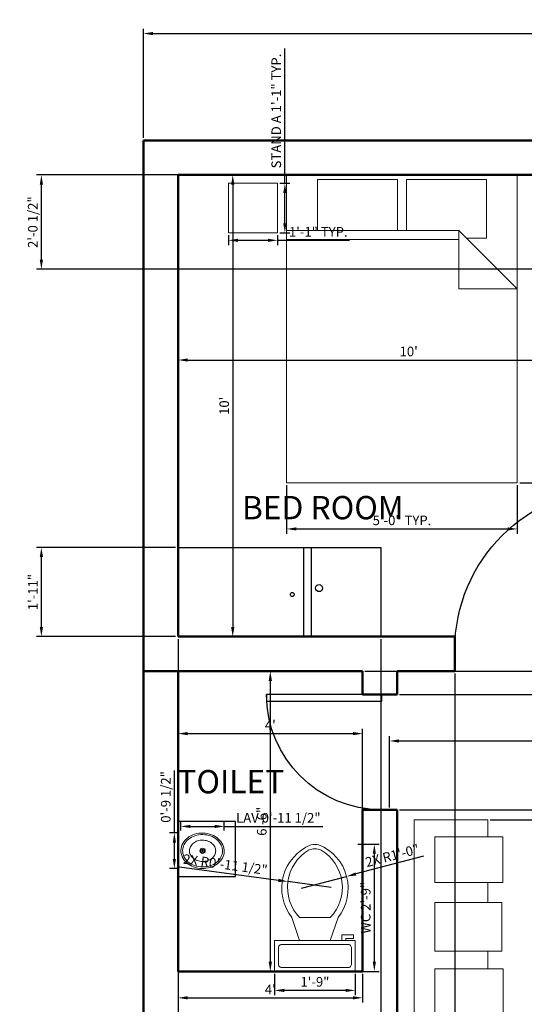
# Model space of a CAD drawing. Units: inches. Extents: x 1071 to 1348, y 2363 to 2916.
# Tile 2 of 4: x 1071 to 1202, y 2660 to 2916. Entities that reach past the tile are written whole.
import ezdxf

# ---------------------------------------------------------------- set-up
doc = ezdxf.new("R2010")
doc.units = ezdxf.units.IN
for name, color, linetype, lineweight in [('A-ANNO-DIMS', 2, 'Continuous', 18), ('A-AREA-IDEN', 7, 'Continuous', 25), ('A-DOOR', 4, 'Continuous', 25), ('A-FLOR-CASE', 9, 'Continuous', 25), ('A-FLOR-FIXT', 9, 'Continuous', 20), ('A-FURN', 8, 'Continuous', 18), ('A-WALL', 7, 'Continuous', 50)]:
    doc.layers.add(name, color=color, linetype=linetype, lineweight=lineweight)
doc.styles.get("Standard").update_dxf_attribs({"font": 'arial.ttf'})
doc.dimstyles.new('ISO-25', dxfattribs={"dimtxt": 2.5, "dimasz": 2.5, "dimexe": 1.25, "dimexo": 0.625, "dimtad": 1, "dimdec": 0, "dimlunit": 3, "dimtxsty": 'Standard', "dimcen": 2.5, "dimadec": 0, "dimazin": 0, "dimtfac": 1, "dimtdec": 0, "dimtmove": 0, "dimatfit": 3, "dimfxl": 1, "dimarcsym": 0})

# ---------------------------------------------------------------- blocks, each defined once
blk = doc.blocks.new('*U2')
for p, q in [((0, 0), (0, -100)), ((750, 0), (750, -100))]:
    blk.add_line(p, q)
blk.add_lwpolyline([(0, 0), (0, 750), (43.75, 750), (43.75, 0)], close=True)
blk.add_arc((0, 0), 750, 0, 90)
blk = doc.blocks.new('Toilet - top')
for p, q in [((9.5, -6), (9.5, -2)), ((-10, -8.5), (-8, -8.5)), ((-10, -9.5), (-10, -8.5)), ((-7, -9.5), (-10, -9.5)), ((-8, -8.5), (-8, -8)), ((-7, -8), (-7, -9.5)), ((-4, -8), (-6, -14)), ((4, -8), (6, -14)), ((4, -14), (-4, -14))]:
    blk.add_line(p, q)
blk.add_lwpolyline([(10.5, -8), (10.5, 0), (-10.5, 0), (-10.5, -8)], close=True)
for points in [[(-9.5, -2), (-9.5, -6)], [(8.5, -1), (-8.5, -1)], [(-8.5, -7), (8.5, -7)]]:
    blk.add_lwpolyline(points)
for centre, radius, start, end in [((-8.62, -1.88), 0.884, 81.8699, 188.1301), ((8.62, -1.88), 0.884, 351.8699, 98.1301), ((-8.62, -6.12), 0.884, 171.8699, 278.1301), ((8.62, -6.12), 0.884, 261.8699, 8.1301), ((3.52, -21.58), 12.17, 141.4691, 247.9714), ((4.2, -21.82), 11.33, 136.3677, 238.9468), ((-3.52, -21.58), 12.17, 292.0284, 38.5307), ((-4.2, -21.82), 11.33, 301.053, 43.6321), ((0, -27.88), 4, 245.7318, 294.2682), ((0, -29), 4, 254.8605, 285.1395)]:
    blk.add_arc(centre, radius, start, end)
blk = doc.blocks.new('Sink - Oval top')
for p, q in [((-1, 0), (1, 0)), ((0, 1), (0, -1))]:
    blk.add_line(p, q)
for points in [[(-12.23, 0.39, 0.117634), (-11.46, -3.36, 0.104469), (-8.88, -6.8, 0.090016), (-5.08, -9.07, 0.08192), (-0.32, -10.02, 0.08192), (4.49, -9.38, 0.090016), (8.42, -7.36, 0.104469), (11.22, -4.09, 0.117634), (12.23, -0.39, 0.117634), (11.46, 3.36, 0.104469), (8.88, 6.8, 0.090016), (5.08, 9.07, 0.08192), (0.32, 10.02, 0.08192), (-4.49, 9.38, 0.090016), (-8.42, 7.36, 0.104469), (-11.22, 4.09, 0.117634)], [(-11.29, 0.16, 0.118622), (-10.52, -3.25, 0.104678), (-8.07, -6.36, 0.089562), (-4.54, -8.37, 0.081185), (-0.13, -9.15, 0.081185), (4.3, -8.49, 0.089562), (7.89, -6.58, 0.104678), (10.42, -3.55, 0.118622), (11.29, -0.16, 0.118622), (10.52, 3.25, 0.104678), (8.07, 6.36, 0.089562), (4.54, 8.37, 0.081185), (0.13, 9.15, 0.081185), (-4.3, 8.49, 0.089562), (-7.89, 6.58, 0.104678), (-10.42, 3.55, 0.118622)], [(-7.42, 0.08, 0.118283), (-6.91, -2.17, 0.104607), (-5.29, -4.21, 0.089718), (-2.97, -5.53, 0.081436), (-0.07, -6.04, 0.081436), (2.84, -5.59, 0.089718), (5.2, -4.33, 0.104607), (6.86, -2.32, 0.118283), (7.42, -0.08, 0.118283), (6.91, 2.17, 0.104607), (5.29, 4.21, 0.089718), (2.97, 5.53, 0.081436), (0.07, 6.04, 0.081436), (-2.84, 5.59, 0.089718), (-5.2, 4.33, 0.104607), (-6.86, 2.32, 0.118283)]]:
    blk.add_lwpolyline(points, format="xyb", close=True)
for radius in [1.5, 1]:
    blk.add_circle((0, 0), radius)
blk = doc.blocks.new('Bed - Queen')
for p, q in [((0, -80.00003), (0, 0)), ((0, 0), (59.99999, 0)), ((59.99999, 0), (59.99999, -80.00003)), ((7.99999, -1.2), (28.79998, -1.2)), ((7.99999, -14.4), (7.99999, -1.2)), ((28.79998, -1.2), (28.79998, -14.4)), ((31.19999, -1.2), (51.99999, -1.2)), ((31.19999, -14.4), (31.19999, -1.2)), ((51.99999, -1.2), (51.99999, -16.4)), ((0, -14.4), (44.8, -14.4)), ((59.99999, -29.6), (44.8, -14.4)), ((44.8, -14.4), (44.8, -29.6)), ((44.8, -16.8), (0, -16.8)), ((51.99999, -16.4), (46.79936, -16.4)), ((44.8, -29.6), (59.99999, -29.6)), ((59.99999, -80.00003), (0, -80.00003))]:
    blk.add_line(p, q)
blk = doc.blocks.new('*D9')
at = {"layer": 'A-ANNO-DIMS', "color": 0, "lineweight": -2, "transparency": 16777216}
for p, q in [((1103.28, 2884.88), (1103.28, 2913.26)), ((1319.28, 2884.88), (1319.28, 2913.26)), ((1105.78, 2912.01), (1316.78, 2912.01))]:
    blk.add_line(p, q, dxfattribs=at)
at = {"layer": 'A-ANNO-DIMS', "color": 0, "transparency": 16777216}
for points in [[(1105.78, 2912.43), (1105.78, 2911.6), (1103.28, 2912.01)], [(1316.78, 2912.43), (1316.78, 2911.6), (1319.28, 2912.01)]]:
    blk.add_solid(points, dxfattribs=at)
at = {"layer": 'Defpoints', "color": 0, "transparency": 16777216}
for p in [(1319.28, 2912.01), (1103.28, 2884.25), (1319.28, 2884.25)]:
    blk.add_point(p, dxfattribs=at)
at = {"layer": 'A-ANNO-DIMS', "color": 0, "transparency": 16777216, "insert": (1211.28, 2913.91), "char_height": 2.5, "attachment_point": 5}
blk.add_mtext("18'", dxfattribs=at)
blk = doc.blocks.new('*D14')
at = {"layer": 'A-ANNO-DIMS', "color": 0, "lineweight": -2, "transparency": 16777216}
for p, q in [((1167.28, 2710.88), (1167.28, 2729.38)), ((1310.28, 2710.88), (1310.28, 2729.38)), ((1169.78, 2728.13), (1307.78, 2728.13))]:
    blk.add_line(p, q, dxfattribs=at)
at = {"layer": 'A-ANNO-DIMS', "color": 0, "transparency": 16777216}
for points in [[(1169.78, 2728.55), (1169.78, 2727.72), (1167.28, 2728.13)], [(1307.78, 2728.55), (1307.78, 2727.72), (1310.28, 2728.13)]]:
    blk.add_solid(points, dxfattribs=at)
at = {"layer": 'Defpoints', "color": 0, "transparency": 16777216}
for p in [(1310.28, 2728.13), (1167.28, 2710.25), (1310.28, 2710.25)]:
    blk.add_point(p, dxfattribs=at)
at = {"layer": 'A-ANNO-DIMS', "color": 0, "transparency": 16777216, "insert": (1238.78, 2730.01), "char_height": 2.5, "attachment_point": 5}
blk.add_mtext('11\'-11"', dxfattribs=at)
blk = doc.blocks.new('*D19')
at = {"layer": 'A-ANNO-DIMS', "color": 0, "lineweight": -2, "transparency": 16777216}
for p, q in [((1112.91, 2746.25), (1137.53, 2746.25)), ((1136.28, 2743.75), (1136.28, 2670.75)), ((1112.91, 2668.25), (1137.53, 2668.25))]:
    blk.add_line(p, q, dxfattribs=at)
at = {"layer": 'A-ANNO-DIMS', "color": 0, "transparency": 16777216}
for points in [[(1135.86, 2743.75), (1136.7, 2743.75), (1136.28, 2746.25)], [(1135.86, 2670.75), (1136.7, 2670.75), (1136.28, 2668.25)]]:
    blk.add_solid(points, dxfattribs=at)
at = {"layer": 'Defpoints', "color": 0, "transparency": 16777216}
for p in [(1112.28, 2746.25), (1112.28, 2668.25), (1136.28, 2668.25)]:
    blk.add_point(p, dxfattribs=at)
at = {"layer": 'A-ANNO-DIMS', "color": 0, "transparency": 16777216, "insert": (1134.38, 2707.25), "char_height": 2.5, "attachment_point": 5, "rotation": 90}
blk.add_mtext('6\'-6"', dxfattribs=at)
blk = doc.blocks.new('*D20')
at = {"layer": 'A-ANNO-DIMS', "color": 0, "lineweight": -2, "transparency": 16777216}
for p, q in [((1112.28, 2668.88), (1112.28, 2731.3)), ((1160.28, 2668.88), (1160.28, 2731.3)), ((1114.78, 2730.05), (1157.78, 2730.05))]:
    blk.add_line(p, q, dxfattribs=at)
at = {"layer": 'A-ANNO-DIMS', "color": 0, "transparency": 16777216}
for points in [[(1114.78, 2730.47), (1114.78, 2729.63), (1112.28, 2730.05)], [(1157.78, 2730.47), (1157.78, 2729.63), (1160.28, 2730.05)]]:
    blk.add_solid(points, dxfattribs=at)
at = {"layer": 'Defpoints', "color": 0, "transparency": 16777216}
for p in [(1160.28, 2730.05), (1112.28, 2668.25), (1160.28, 2668.25)]:
    blk.add_point(p, dxfattribs=at)
at = {"layer": 'A-ANNO-DIMS', "color": 0, "transparency": 16777216, "insert": (1136.28, 2731.93), "char_height": 2.5, "attachment_point": 5}
blk.add_mtext("4'", dxfattribs=at)
blk = doc.blocks.new('*D24')
at = {"layer": 'A-ANNO-DIMS', "color": 0, "lineweight": -2, "transparency": 16777216}
for p, q in [((1112.28, 2874.63), (1112.28, 2825.9)), ((1232.28, 2874.63), (1232.28, 2825.9)), ((1114.78, 2827.15), (1229.78, 2827.15))]:
    blk.add_line(p, q, dxfattribs=at)
at = {"layer": 'A-ANNO-DIMS', "color": 0, "transparency": 16777216}
for points in [[(1114.78, 2827.57), (1114.78, 2826.74), (1112.28, 2827.15)], [(1229.78, 2827.57), (1229.78, 2826.74), (1232.28, 2827.15)]]:
    blk.add_solid(points, dxfattribs=at)
at = {"layer": 'Defpoints', "color": 0, "transparency": 16777216}
for p in [(1112.28, 2875.25), (1232.28, 2875.25), (1232.28, 2827.15)]:
    blk.add_point(p, dxfattribs=at)
at = {"layer": 'A-ANNO-DIMS', "color": 0, "transparency": 16777216, "insert": (1172.28, 2829.06), "char_height": 2.5, "attachment_point": 5}
blk.add_mtext("10'", dxfattribs=at)
blk = doc.blocks.new('*D25')
at = {"layer": 'A-ANNO-DIMS', "color": 0, "lineweight": -2, "transparency": 16777216}
for p, q in [((1112.91, 2875.25), (1127.76, 2875.25)), ((1126.51, 2872.75), (1126.51, 2757.75)), ((1112.91, 2755.25), (1127.76, 2755.25))]:
    blk.add_line(p, q, dxfattribs=at)
at = {"layer": 'A-ANNO-DIMS', "color": 0, "transparency": 16777216}
for points in [[(1126.09, 2872.75), (1126.93, 2872.75), (1126.51, 2875.25)], [(1126.09, 2757.75), (1126.93, 2757.75), (1126.51, 2755.25)]]:
    blk.add_solid(points, dxfattribs=at)
at = {"layer": 'Defpoints', "color": 0, "transparency": 16777216}
for p in [(1112.28, 2875.25), (1112.28, 2755.25), (1126.51, 2755.25)]:
    blk.add_point(p, dxfattribs=at)
at = {"layer": 'A-ANNO-DIMS', "color": 0, "transparency": 16777216, "insert": (1124.61, 2815.25), "char_height": 2.5, "attachment_point": 5, "rotation": 90}
blk.add_mtext("10'", dxfattribs=at)
blk = doc.blocks.new('*D26')
at = {"layer": 'A-ANNO-DIMS', "color": 0, "lineweight": -2, "transparency": 16777216}
for p, q in [((1112.28, 2667.63), (1112.28, 2660.12)), ((1160.28, 2667.63), (1160.28, 2660.12)), ((1114.78, 2661.37), (1157.78, 2661.37))]:
    blk.add_line(p, q, dxfattribs=at)
at = {"layer": 'A-ANNO-DIMS', "color": 0, "transparency": 16777216}
for points in [[(1114.78, 2661.78), (1114.78, 2660.95), (1112.28, 2661.37)], [(1157.78, 2661.78), (1157.78, 2660.95), (1160.28, 2661.37)]]:
    blk.add_solid(points, dxfattribs=at)
at = {"layer": 'Defpoints', "color": 0, "transparency": 16777216}
for p in [(1112.28, 2668.25), (1160.28, 2668.25), (1160.28, 2661.37)]:
    blk.add_point(p, dxfattribs=at)
at = {"layer": 'A-ANNO-DIMS', "color": 0, "transparency": 16777216, "insert": (1136.28, 2663.24), "char_height": 2.5, "attachment_point": 5}
blk.add_mtext("4'", dxfattribs=at)
blk = doc.blocks.new('NIGHTSTAND-A')
blk.add_lwpolyline([(0, 12.88), (12.76, 12.88), (12.76, 0), (0, 0)], close=True)
blk = doc.blocks.new('*D29')
at = {"layer": 'A-ANNO-DIMS', "color": 0, "lineweight": -2, "transparency": 16777216}
for p, q in [((1201.15, 2875.25), (1213.78, 2875.25)), ((1212.53, 2797.75), (1212.53, 2872.75)), ((1201.15, 2795.25), (1213.78, 2795.25))]:
    blk.add_line(p, q, dxfattribs=at)
at = {"layer": 'A-ANNO-DIMS', "color": 0, "transparency": 16777216}
for points in [[(1212.11, 2872.75), (1212.94, 2872.75), (1212.53, 2875.25)], [(1212.11, 2797.75), (1212.94, 2797.75), (1212.53, 2795.25)]]:
    blk.add_solid(points, dxfattribs=at)
at = {"layer": 'Defpoints', "color": 0, "transparency": 16777216}
for p in [(1200.53, 2875.25), (1212.53, 2875.25), (1200.53, 2795.25)]:
    blk.add_point(p, dxfattribs=at)
at = {"layer": 'A-ANNO-DIMS', "color": 0, "transparency": 16777216, "insert": (1210.62, 2835.25), "char_height": 2.5, "attachment_point": 5, "rotation": 90}
blk.add_mtext('BED 6\'-8" TYP.', dxfattribs=at)
blk = doc.blocks.new('*D30')
at = {"layer": 'A-ANNO-DIMS', "color": 0, "lineweight": -2, "transparency": 16777216}
for p, q in [((1140.53, 2794.63), (1140.53, 2782)), ((1200.53, 2794.63), (1200.53, 2782)), ((1143.03, 2783.25), (1198.03, 2783.25))]:
    blk.add_line(p, q, dxfattribs=at)
at = {"layer": 'A-ANNO-DIMS', "color": 0, "transparency": 16777216}
for points in [[(1143.03, 2783.67), (1143.03, 2782.84), (1140.53, 2783.25)], [(1198.03, 2783.67), (1198.03, 2782.84), (1200.53, 2783.25)]]:
    blk.add_solid(points, dxfattribs=at)
at = {"layer": 'Defpoints', "color": 0, "transparency": 16777216}
for p in [(1140.53, 2795.25), (1200.53, 2795.25), (1200.53, 2783.25)]:
    blk.add_point(p, dxfattribs=at)
at = {"layer": 'A-ANNO-DIMS', "color": 0, "transparency": 16777216, "insert": (1170.53, 2785.16), "char_height": 2.5, "attachment_point": 5}
blk.add_mtext('5\'-0" TYP.', dxfattribs=at)
blk = doc.blocks.new('*D31')
at = {"layer": 'A-ANNO-DIMS', "color": 0, "lineweight": -2, "transparency": 16777216}
for p, q in [((1140.07, 2873.09), (1140.07, 2908.17)), ((1138.76, 2873.09), (1141.32, 2873.09)), ((1140.07, 2862.71), (1140.07, 2870.59)), ((1138.76, 2860.21), (1141.32, 2860.21))]:
    blk.add_line(p, q, dxfattribs=at)
at = {"layer": 'A-ANNO-DIMS', "color": 0, "transparency": 16777216}
for points in [[(1139.65, 2870.59), (1140.49, 2870.59), (1140.07, 2873.09)], [(1139.65, 2862.71), (1140.49, 2862.71), (1140.07, 2860.21)]]:
    blk.add_solid(points, dxfattribs=at)
at = {"layer": 'Defpoints', "color": 0, "transparency": 16777216}
for p in [(1138.14, 2873.09), (1140.07, 2873.09), (1138.14, 2860.21)]:
    blk.add_point(p, dxfattribs=at)
at = {"layer": 'A-ANNO-DIMS', "color": 0, "transparency": 16777216, "insert": (1138.15, 2891.88), "char_height": 2.5, "attachment_point": 5, "rotation": 90}
blk.add_mtext('STAND A 1\'-1" TYP.', dxfattribs=at)
blk = doc.blocks.new('*D32')
at = {"layer": 'A-ANNO-DIMS', "color": 0, "lineweight": -2, "transparency": 16777216}
for p, q in [((1125.38, 2859.58), (1125.38, 2857.02)), ((1138.14, 2859.58), (1138.14, 2857.02)), ((1127.88, 2858.27), (1135.64, 2858.27)), ((1138.14, 2858.27), (1156.89, 2858.27))]:
    blk.add_line(p, q, dxfattribs=at)
at = {"layer": 'A-ANNO-DIMS', "color": 0, "transparency": 16777216}
for points in [[(1127.88, 2858.69), (1127.88, 2857.86), (1125.38, 2858.27)], [(1135.64, 2858.69), (1135.64, 2857.86), (1138.14, 2858.27)]]:
    blk.add_solid(points, dxfattribs=at)
at = {"layer": 'Defpoints', "color": 0, "transparency": 16777216}
for p in [(1125.38, 2860.21), (1138.14, 2860.21), (1138.14, 2858.27)]:
    blk.add_point(p, dxfattribs=at)
at = {"layer": 'A-ANNO-DIMS', "color": 0, "transparency": 16777216, "insert": (1148.76, 2860.15), "char_height": 2.5, "attachment_point": 5}
blk.add_mtext('1\'-1" TYP.', dxfattribs=at)
blk = doc.blocks.new('*D35')
at = {"layer": 'A-ANNO-DIMS', "color": 0, "lineweight": -2, "transparency": 16777216}
for p, q in [((1159.01, 2701.3), (1164.59, 2701.3)), ((1163.34, 2698.8), (1163.34, 2670.75)), ((1159.01, 2668.25), (1164.59, 2668.25))]:
    blk.add_line(p, q, dxfattribs=at)
at = {"layer": 'A-ANNO-DIMS', "color": 0, "transparency": 16777216}
for points in [[(1162.93, 2698.8), (1163.76, 2698.8), (1163.34, 2701.3)], [(1162.93, 2670.75), (1163.76, 2670.75), (1163.34, 2668.25)]]:
    blk.add_solid(points, dxfattribs=at)
at = {"layer": 'Defpoints', "color": 0, "transparency": 16777216}
for p in [(1158.39, 2701.3), (1158.39, 2668.25), (1163.34, 2668.25)]:
    blk.add_point(p, dxfattribs=at)
at = {"layer": 'A-ANNO-DIMS', "color": 0, "transparency": 16777216, "insert": (1161.42, 2684.78), "char_height": 2.5, "attachment_point": 5, "rotation": 90}
blk.add_mtext('WC 2\'-9"', dxfattribs=at)
blk = doc.blocks.new('*D36')
at = {"layer": 'A-ANNO-DIMS', "color": 0, "lineweight": -2, "transparency": 16777216}
for p, q in [((1137.39, 2667.63), (1137.39, 2662.05)), ((1158.39, 2667.63), (1158.39, 2662.05)), ((1155.89, 2663.3), (1139.89, 2663.3))]:
    blk.add_line(p, q, dxfattribs=at)
at = {"layer": 'A-ANNO-DIMS', "color": 0, "transparency": 16777216}
for points in [[(1139.89, 2663.71), (1139.89, 2662.88), (1137.39, 2663.3)], [(1155.89, 2663.71), (1155.89, 2662.88), (1158.39, 2663.3)]]:
    blk.add_solid(points, dxfattribs=at)
at = {"layer": 'Defpoints', "color": 0, "transparency": 16777216}
for p in [(1137.39, 2668.25), (1158.39, 2668.25), (1137.39, 2663.3)]:
    blk.add_point(p, dxfattribs=at)
at = {"layer": 'A-ANNO-DIMS', "color": 0, "transparency": 16777216, "insert": (1147.89, 2665.2), "char_height": 2.5, "attachment_point": 5}
blk.add_mtext('1\'-9"', dxfattribs=at)
blk = doc.blocks.new('*D37')
at = {"layer": 'A-ANNO-DIMS', "color": 0, "lineweight": -2, "transparency": 16777216}
for p, q in [((1113.02, 2704.85), (1113.02, 2707.17)), ((1115.52, 2705.92), (1121.81, 2705.92)), ((1124.31, 2704.85), (1124.31, 2707.17)), ((1124.31, 2705.92), (1149.93, 2705.92))]:
    blk.add_line(p, q, dxfattribs=at)
at = {"layer": 'A-ANNO-DIMS', "color": 0, "transparency": 16777216}
for points in [[(1115.52, 2706.34), (1115.52, 2705.5), (1113.02, 2705.92)], [(1121.81, 2706.34), (1121.81, 2705.5), (1124.31, 2705.92)]]:
    blk.add_solid(points, dxfattribs=at)
at = {"layer": 'Defpoints', "color": 0, "transparency": 16777216}
for p in [(1124.31, 2705.92), (1113.02, 2704.23), (1124.31, 2704.23)]:
    blk.add_point(p, dxfattribs=at)
at = {"layer": 'A-ANNO-DIMS', "color": 0, "transparency": 16777216, "insert": (1138.37, 2707.84), "char_height": 2.5, "attachment_point": 5}
blk.add_mtext('LAV 0\'-11 1/2"', dxfattribs=at)
blk = doc.blocks.new('*D38')
at = {"layer": 'A-ANNO-DIMS', "color": 0, "lineweight": -2, "transparency": 16777216}
for p, q in [((1111.32, 2704.23), (1111.32, 2720.45)), ((1112.39, 2704.23), (1110.07, 2704.23)), ((1111.32, 2697.46), (1111.32, 2701.73)), ((1112.39, 2694.96), (1110.07, 2694.96))]:
    blk.add_line(p, q, dxfattribs=at)
at = {"layer": 'A-ANNO-DIMS', "color": 0, "transparency": 16777216}
for points in [[(1110.91, 2701.73), (1111.74, 2701.73), (1111.32, 2704.23)], [(1110.91, 2697.46), (1111.74, 2697.46), (1111.32, 2694.96)]]:
    blk.add_solid(points, dxfattribs=at)
at = {"layer": 'Defpoints', "color": 0, "transparency": 16777216}
for p in [(1111.32, 2704.23), (1113.02, 2704.23), (1113.02, 2694.96)]:
    blk.add_point(p, dxfattribs=at)
at = {"layer": 'A-ANNO-DIMS', "color": 0, "transparency": 16777216, "insert": (1109.41, 2713.59), "char_height": 2.5, "attachment_point": 5, "rotation": 90}
blk.add_mtext('0\'-9 1/2"', dxfattribs=at)
blk = doc.blocks.new('*D48')
at = {"layer": 'A-ANNO-DIMS', "color": 0, "lineweight": -2, "transparency": 16777216}
for p, q in [((1184.28, 2745.63), (1184.28, 2363.45)), ((1226.28, 2745.63), (1226.28, 2363.45)), ((1186.78, 2364.7), (1223.78, 2364.7))]:
    blk.add_line(p, q, dxfattribs=at)
at = {"layer": 'A-ANNO-DIMS', "color": 0, "transparency": 16777216}
for points in [[(1186.78, 2365.12), (1186.78, 2364.29), (1184.28, 2364.7)], [(1223.78, 2365.12), (1223.78, 2364.29), (1226.28, 2364.7)]]:
    blk.add_solid(points, dxfattribs=at)
at = {"layer": 'Defpoints', "color": 0, "transparency": 16777216}
for p in [(1184.28, 2746.25), (1226.28, 2746.25), (1226.28, 2364.7)]:
    blk.add_point(p, dxfattribs=at)
at = {"layer": 'A-ANNO-DIMS', "color": 0, "transparency": 16777216, "insert": (1205.28, 2366.61), "char_height": 2.5, "attachment_point": 5}
blk.add_mtext('3\'-6"', dxfattribs=at)
blk = doc.blocks.new('*D50')
at = {"layer": 'A-ANNO-DIMS', "color": 0, "lineweight": -2, "transparency": 16777216}
for p, q in [((1169.91, 2740.25), (1347.08, 2740.25)), ((1345.83, 2737.75), (1345.83, 2712.75)), ((1169.91, 2710.25), (1347.08, 2710.25))]:
    blk.add_line(p, q, dxfattribs=at)
at = {"layer": 'A-ANNO-DIMS', "color": 0, "transparency": 16777216}
for points in [[(1345.41, 2737.75), (1346.25, 2737.75), (1345.83, 2740.25)], [(1345.41, 2712.75), (1346.25, 2712.75), (1345.83, 2710.25)]]:
    blk.add_solid(points, dxfattribs=at)
at = {"layer": 'Defpoints', "color": 0, "transparency": 16777216}
for p in [(1169.28, 2740.25), (1169.28, 2710.25), (1345.83, 2710.25)]:
    blk.add_point(p, dxfattribs=at)
at = {"layer": 'A-ANNO-DIMS', "color": 0, "transparency": 16777216, "insert": (1343.93, 2725.25), "char_height": 2.5, "attachment_point": 5, "rotation": 90}
blk.add_mtext('2\'-6"', dxfattribs=at)
blk = doc.blocks.new('*D52')
at = {"layer": 'A-ANNO-DIMS', "color": 0, "lineweight": -2, "transparency": 16777216}
for p, q in [((1345.83, 2748.75), (1345.83, 2759.15)), ((1160.91, 2746.25), (1347.08, 2746.25)), ((1345.83, 2740.25), (1345.83, 2746.25)), ((1169.91, 2740.25), (1347.08, 2740.25)), ((1345.83, 2737.75), (1345.83, 2735.25))]:
    blk.add_line(p, q, dxfattribs=at)
at = {"layer": 'A-ANNO-DIMS', "color": 0, "transparency": 16777216}
for points in [[(1345.41, 2748.75), (1346.25, 2748.75), (1345.83, 2746.25)], [(1345.41, 2737.75), (1346.25, 2737.75), (1345.83, 2740.25)]]:
    blk.add_solid(points, dxfattribs=at)
at = {"layer": 'Defpoints', "color": 0, "transparency": 16777216}
for p in [(1160.28, 2746.25), (1345.83, 2746.25), (1169.28, 2740.25)]:
    blk.add_point(p, dxfattribs=at)
at = {"layer": 'A-ANNO-DIMS', "color": 0, "transparency": 16777216, "insert": (1343.93, 2755.2), "char_height": 2.5, "attachment_point": 5, "rotation": 90}
blk.add_mtext('0\'-6"', dxfattribs=at)
blk = doc.blocks.new('*D62')
at = {"layer": 'A-ANNO-DIMS', "color": 0, "lineweight": -2, "transparency": 16777216}
for p, q in [((1240.66, 2875.25), (1075.48, 2875.25)), ((1076.73, 2853.23), (1076.73, 2872.75)), ((1240.66, 2850.73), (1075.48, 2850.73))]:
    blk.add_line(p, q, dxfattribs=at)
at = {"layer": 'A-ANNO-DIMS', "color": 0, "transparency": 16777216}
for points in [[(1076.31, 2872.75), (1077.15, 2872.75), (1076.73, 2875.25)], [(1076.31, 2853.23), (1077.15, 2853.23), (1076.73, 2850.73)]]:
    blk.add_solid(points, dxfattribs=at)
at = {"layer": 'Defpoints', "color": 0, "transparency": 16777216}
for p in [(1076.73, 2875.25), (1241.28, 2875.25), (1241.28, 2850.73)]:
    blk.add_point(p, dxfattribs=at)
at = {"layer": 'A-ANNO-DIMS', "color": 0, "transparency": 16777216, "insert": (1074.81, 2862.99), "char_height": 2.5, "attachment_point": 5, "rotation": 90}
blk.add_mtext('2\'-0 1/2"', dxfattribs=at)
blk = doc.blocks.new('*D63')
at = {"layer": 'A-ANNO-DIMS', "color": 0, "lineweight": -2, "transparency": 16777216}
for p, q in [((1112.28, 2754.63), (1112.28, 2363.45)), ((1165.02, 2754.63), (1165.02, 2363.45)), ((1114.78, 2364.7), (1162.52, 2364.7))]:
    blk.add_line(p, q, dxfattribs=at)
at = {"layer": 'A-ANNO-DIMS', "color": 0, "transparency": 16777216}
for points in [[(1114.78, 2365.12), (1114.78, 2364.29), (1112.28, 2364.7)], [(1162.52, 2365.12), (1162.52, 2364.29), (1165.02, 2364.7)]]:
    blk.add_solid(points, dxfattribs=at)
at = {"layer": 'Defpoints', "color": 0, "transparency": 16777216}
for p in [(1112.28, 2755.25), (1165.02, 2755.25), (1165.02, 2364.7)]:
    blk.add_point(p, dxfattribs=at)
at = {"layer": 'A-ANNO-DIMS', "color": 0, "transparency": 16777216, "insert": (1138.65, 2366.62), "char_height": 2.5, "attachment_point": 5}
blk.add_mtext('4\'-4 1/2"', dxfattribs=at)
blk = doc.blocks.new('*D64')
at = {"layer": 'A-ANNO-DIMS', "color": 0, "lineweight": -2, "transparency": 16777216}
for p, q in [((1111.66, 2778.43), (1075.48, 2778.43)), ((1076.73, 2757.75), (1076.73, 2775.93)), ((1111.66, 2755.25), (1075.48, 2755.25))]:
    blk.add_line(p, q, dxfattribs=at)
at = {"layer": 'A-ANNO-DIMS', "color": 0, "transparency": 16777216}
for points in [[(1076.31, 2775.93), (1077.15, 2775.93), (1076.73, 2778.43)], [(1076.31, 2757.75), (1077.15, 2757.75), (1076.73, 2755.25)]]:
    blk.add_solid(points, dxfattribs=at)
at = {"layer": 'Defpoints', "color": 0, "transparency": 16777216}
for p in [(1076.73, 2778.43), (1112.28, 2778.43), (1112.28, 2755.25)]:
    blk.add_point(p, dxfattribs=at)
at = {"layer": 'A-ANNO-DIMS', "color": 0, "transparency": 16777216, "insert": (1074.85, 2766.84), "char_height": 2.5, "attachment_point": 5, "rotation": 90}
blk.add_mtext('1\'-11"', dxfattribs=at)
blk = doc.blocks.new('*D66')
at = {"layer": 'A-ANNO-DIMS', "color": 0, "lineweight": -2, "transparency": 16777216}
for p, q in [((1193.46, 2707.65), (1347.08, 2707.65)), ((1345.83, 2705.15), (1345.83, 2639.07)), ((1216.75, 2636.57), (1347.08, 2636.57))]:
    blk.add_line(p, q, dxfattribs=at)
at = {"layer": 'A-ANNO-DIMS', "color": 0, "transparency": 16777216}
for points in [[(1345.41, 2705.15), (1346.25, 2705.15), (1345.83, 2707.65)], [(1345.41, 2639.07), (1346.25, 2639.07), (1345.83, 2636.57)]]:
    blk.add_solid(points, dxfattribs=at)
at = {"layer": 'Defpoints', "color": 0, "transparency": 16777216}
for p in [(1192.84, 2707.65), (1216.12, 2636.57), (1345.83, 2636.57)]:
    blk.add_point(p, dxfattribs=at)
at = {"layer": 'A-ANNO-DIMS', "color": 0, "transparency": 16777216, "insert": (1343.93, 2672.11), "char_height": 2.5, "attachment_point": 5, "rotation": 90}
blk.add_mtext('5\'-11"', dxfattribs=at)
blk = doc.blocks.new('*D69')
at = {"layer": 'A-ANNO-DIMS', "color": 0, "lineweight": -2, "transparency": 16777216}
for p, q in [((1176.16, 2698.19), (1158.55, 2693.56)), ((1144.37, 2689.84), (1156.14, 2692.93))]:
    blk.add_line(p, q, dxfattribs=at)
at = {"layer": 'A-ANNO-DIMS', "color": 0, "transparency": 16777216}
blk.add_solid([(1158.45, 2693.97), (1158.66, 2693.16), (1156.14, 2692.93)], dxfattribs=at)
at = {"layer": 'Defpoints', "color": 0, "transparency": 16777216}
for p in [(1156.14, 2692.93), (1144.37, 2689.84)]:
    blk.add_point(p, dxfattribs=at)
at = {"layer": 'A-ANNO-DIMS', "color": 0, "transparency": 16777216, "insert": (1168.08, 2698.03), "char_height": 2.5, "attachment_point": 5, "rotation": 14.718}
blk.add_mtext('2X R1\'-0"', dxfattribs=at)
blk = doc.blocks.new('*D70')
at = {"layer": 'A-ANNO-DIMS', "color": 0, "lineweight": -2, "transparency": 16777216}
for p, q in [((1112.64, 2695.38), (1138.38, 2691.92)), ((1152.09, 2690.07), (1140.86, 2691.58))]:
    blk.add_line(p, q, dxfattribs=at)
at = {"layer": 'A-ANNO-DIMS', "color": 0, "transparency": 16777216}
blk.add_solid([(1138.44, 2692.33), (1138.32, 2691.5), (1140.86, 2691.58)], dxfattribs=at)
at = {"layer": 'Defpoints', "color": 0, "transparency": 16777216}
for p in [(1140.86, 2691.58), (1152.09, 2690.07)]:
    blk.add_point(p, dxfattribs=at)
at = {"layer": 'A-ANNO-DIMS', "color": 0, "transparency": 16777216, "insert": (1124.53, 2695.71), "char_height": 2.5, "attachment_point": 5, "rotation": 352.3417}
blk.add_mtext('2X R0\'-11 1/2"', dxfattribs=at)

msp = doc.modelspace()

# ---------------------------------------------------------------- linework, layer by layer
at = {"layer": 'A-FLOR-CASE'}
for p, q in [((1144.88, 2778.43), (1144.88, 2755.25)), ((1146.88, 2778.43), (1146.88, 2755.25)), ((1127.21, 2707.22), (1112.28, 2707.22)), ((1127.21, 2692.92), (1127.21, 2707.22)), ((1112.28, 2692.92), (1127.21, 2692.92))]:
    msp.add_line(p, q, dxfattribs=at)
msp.add_lwpolyline([(1112.28, 2778.43), (1165.02, 2778.43), (1165.02, 2755.25), (1112.28, 2755.25)], close=True, dxfattribs=at)
for centre, radius in [((1141.98, 2766.21), 0.525), ((1148.96, 2767.86), 0.915)]:
    msp.add_circle(centre, radius, dxfattribs=at)
at = {"layer": 'A-FURN'}
for points in [[(1173.73, 2638.54), (1173.73, 2707.65), (1192.84, 2707.65), (1192.84, 2703.25)], [(1192.84, 2691.31), (1192.84, 2686.12)], [(1192.84, 2673.46), (1192.84, 2668.91)]]:
    msp.add_lwpolyline(points, dxfattribs=at)
for points in [[(1179.12, 2691.31), (1196.77, 2691.31), (1196.77, 2703.25), (1179.12, 2703.25)], [(1179.12, 2673.46), (1196.47, 2673.46), (1196.47, 2686.12), (1179.12, 2686.12)], [(1179.12, 2655.98), (1196.89, 2655.98), (1196.89, 2668.91), (1179.12, 2668.91)]]:
    msp.add_lwpolyline(points, close=True, dxfattribs=at)
at = {"layer": 'A-WALL'}
for p, q in [((1103.28, 2884.25), (1319.28, 2884.25)), ((1103.28, 2884.25), (1103.28, 2391.25)), ((1112.28, 2875.25), (1112.28, 2755.25)), ((1112.28, 2875.25), (1232.28, 2875.25)), ((1112.28, 2755.25), (1184.28, 2755.25)), ((1184.28, 2755.25), (1184.28, 2746.25)), ((1103.28, 2746.25), (1160.28, 2746.25)), ((1112.28, 2746.25), (1112.28, 2668.25)), ((1160.28, 2746.25), (1160.28, 2740.25)), ((1169.28, 2746.25), (1169.28, 2740.25)), ((1169.28, 2746.25), (1184.28, 2746.25)), ((1160.28, 2740.25), (1169.28, 2740.25)), ((1160.28, 2710.25), (1169.28, 2710.25)), ((1160.28, 2710.25), (1160.28, 2668.25)), ((1169.28, 2710.25), (1169.28, 2635.25)), ((1112.28, 2668.25), (1160.28, 2668.25))]:
    msp.add_line(p, q, dxfattribs=at)

# ---------------------------------------------------------------- block references
at = {"layer": 'A-DOOR', "xscale": -0.0559999999999998, "yscale": 0.0559999999999998, "zscale": 0.0559999999999998}
msp.add_blockref('*U2', (1226.28, 2751.85), dxfattribs=at)
at = {"layer": 'A-DOOR', "xscale": -0.04, "yscale": 0.04, "zscale": 0.04, "rotation": 90}
msp.add_blockref('*U2', (1165.28, 2740.25), dxfattribs=at)
at = {"layer": 'A-FLOR-FIXT', "xscale": 0.4599112924858537, "yscale": 0.4599112924858537, "zscale": 0.4599112924858537}
msp.add_blockref('Sink - Oval top', (1118.66, 2699.59), dxfattribs=at)
at = {"layer": 'A-FLOR-FIXT', "rotation": 180}
msp.add_blockref('Toilet - top', (1147.89, 2668.25), dxfattribs=at)
at = {"layer": 'A-FURN'}
for name, p in [('Bed - Queen', (1140.53, 2875.25)), ('NIGHTSTAND-A', (1125.38, 2860.21))]:
    msp.add_blockref(name, p, dxfattribs=at)

# ---------------------------------------------------------------- texts
at = {"layer": 'A-AREA-IDEN'}
for s, p in [('BED ROOM', (1128.92, 2785.76)), ('TOILET', (1112.11, 2714.53))]:
    msp.add_text(s, height=6.055, dxfattribs=at).set_placement(p)

# ---------------------------------------------------------------- dimensions: what is measured, and where the dimension line sits
at = {"layer": 'A-ANNO-DIMS'}
for base, p1, p2, override, picture, middle in [((1319.28, 2912.01), (1103.28, 2884.25), (1319.28, 2884.25), {"dimclrd": 0, "dimclre": 0, "dimclrt": 0}, '*D9', (1211.28, 2913.91)), ((1232.28, 2827.15), (1112.28, 2875.25), (1232.28, 2875.25), {"dimclrd": 0, "dimclre": 0, "dimclrt": 0}, '*D24', (1172.28, 2829.06)), ((1165.02, 2364.7), (1112.28, 2755.25), (1165.02, 2755.25), {"dimdec": 1, "dimlfac": 1, "dimrnd": 0, "dimzin": 1, "dimdsep": 46, "dimlunit": 4, "dimfrac": 2}, '*D63', (1138.65, 2366.62)), ((1226.28, 2364.7), (1184.28, 2746.25), (1226.28, 2746.25), {"dimdec": 1, "dimlfac": 1, "dimrnd": 0, "dimzin": 1, "dimdsep": 46, "dimlunit": 4, "dimfrac": 2}, '*D48', (1205.28, 2366.61)), ((1160.28, 2730.05), (1112.28, 2668.25), (1160.28, 2668.25), {"dimclrd": 0, "dimclre": 0, "dimclrt": 0}, '*D20', (1136.28, 2731.93)), ((1310.28, 2728.13), (1167.28, 2710.25), (1310.28, 2710.25), {"dimclrd": 0, "dimclre": 0, "dimclrt": 0}, '*D14', (1238.78, 2730.01)), ((1160.28, 2661.37), (1112.28, 2668.25), (1160.28, 2668.25), {"dimclrd": 0, "dimclre": 0, "dimclrt": 0}, '*D26', (1136.28, 2663.24))]:
    dim = msp.add_linear_dim(base=base, p1=p1, p2=p2, dimstyle='ISO-25', override=override, dxfattribs=at)
    dim.commit()
    dim.dimension.update_dxf_attribs({"geometry": picture, "text_midpoint": middle})
for base, p1, p2, angle, text, picture, middle in [((1140.07, 2873.09), (1138.14, 2860.21), (1138.14, 2873.09), 90, 'STAND A <> TYP.', '*D31', (1138.15, 2891.88)), ((1212.53, 2875.25), (1200.53, 2795.25), (1200.53, 2875.25), 90, 'BED <> TYP.', '*D29', (1210.62, 2835.25)), ((1163.3426, 2668.2548), (1158.3856, 2701.301), (1158.3856, 2668.2548), 270, 'WC <>', '*D35', (1161.4249, 2684.7779))]:
    dim = msp.add_linear_dim(base=base, p1=p1, p2=p2, angle=angle, text=text, dimstyle='ISO-25', override={"dimdec": 1, "dimlfac": 1, "dimrnd": 0, "dimzin": 1, "dimdsep": 46, "dimlunit": 4, "dimfrac": 2}, dxfattribs=at)
    dim.commit()
    dim.dimension.update_dxf_attribs({"geometry": picture, "text_midpoint": middle})
for base, p1, p2, angle, override, picture, middle in [((1076.73, 2875.25), (1241.28, 2850.73), (1241.28, 2875.25), 90, {"dimdec": 1, "dimlfac": 1, "dimrnd": 0, "dimzin": 1, "dimdsep": 46, "dimlunit": 4, "dimfrac": 2}, '*D62', (1074.81, 2862.99)), ((1126.51, 2755.25), (1112.28, 2875.25), (1112.28, 2755.25), 90, {"dimclrd": 0, "dimclre": 0, "dimclrt": 0}, '*D25', (1124.61, 2815.25)), ((1076.73, 2778.43), (1112.28, 2755.25), (1112.28, 2778.43), 90, {"dimdec": 1, "dimlfac": 1, "dimrnd": 0, "dimzin": 1, "dimdsep": 46, "dimlunit": 4, "dimfrac": 2}, '*D64', (1074.85, 2766.84)), ((1345.83, 2746.25), (1169.28, 2740.25), (1160.28, 2746.25), 90, {"dimdec": 1, "dimlfac": 1, "dimrnd": 0, "dimzin": 1, "dimdsep": 46, "dimlunit": 4, "dimfrac": 2}, '*D52', (1343.93, 2755.2)), ((1136.28, 2668.25), (1112.28, 2746.25), (1112.28, 2668.25), 90, {"dimclrd": 0, "dimclre": 0, "dimclrt": 0}, '*D19', (1134.38, 2707.25)), ((1345.83, 2710.25), (1169.28, 2740.25), (1169.28, 2710.25), 90, {"dimdec": 1, "dimlfac": 1, "dimrnd": 0, "dimzin": 1, "dimdsep": 46, "dimlunit": 4, "dimfrac": 2}, '*D50', (1343.93, 2725.25)), ((1111.32, 2704.23), (1113.02, 2694.96), (1113.02, 2704.23), 90, {"dimdec": 1, "dimlfac": 1, "dimrnd": 0, "dimzin": 1, "dimdsep": 46, "dimlunit": 4, "dimfrac": 2}, '*D38', (1109.41, 2713.59)), ((1345.83, 2636.57), (1192.84, 2707.65), (1216.12, 2636.57), 90, {"dimdec": 1, "dimlfac": 1, "dimrnd": 0, "dimzin": 1, "dimdsep": 46, "dimlunit": 4, "dimfrac": 2}, '*D66', (1343.93, 2672.11)), ((1137.39, 2663.3), (1158.39, 2668.25), (1137.39, 2668.25), 180, {"dimdec": 1, "dimlfac": 1, "dimrnd": 0, "dimzin": 1, "dimdsep": 46, "dimlunit": 4, "dimfrac": 2}, '*D36', (1147.89, 2665.2))]:
    dim = msp.add_linear_dim(base=base, p1=p1, p2=p2, angle=angle, dimstyle='ISO-25', override=override, dxfattribs=at)
    dim.commit()
    dim.dimension.update_dxf_attribs({"geometry": picture, "text_midpoint": middle})
for base, p1, p2, text, picture, middle in [((1138.14, 2858.27), (1125.38, 2860.21), (1138.14, 2860.21), '<> TYP.', '*D32', (1148.76, 2860.15)), ((1200.53, 2783.25), (1140.53, 2795.25), (1200.53, 2795.25), '<> TYP.', '*D30', (1170.53, 2785.16)), ((1124.31, 2705.92), (1113.02, 2704.23), (1124.31, 2704.23), 'LAV <>', '*D37', (1138.37, 2707.84))]:
    dim = msp.add_linear_dim(base=base, p1=p1, p2=p2, text=text, dimstyle='ISO-25', override={"dimdec": 1, "dimlfac": 1, "dimrnd": 0, "dimzin": 1, "dimdsep": 46, "dimlunit": 4, "dimfrac": 2}, dxfattribs=at)
    dim.commit()
    dim.dimension.update_dxf_attribs({"geometry": picture, "text_midpoint": middle})
for center, mpoint, picture, middle in [((1144.37, 2689.84), (1156.14, 2692.93), '*D69', (1168.08, 2698.03)), ((1152.09, 2690.07), (1140.86, 2691.58), '*D70', (1124.53, 2695.71))]:
    dim = msp.add_radius_dim(center=center, mpoint=mpoint, text='2X <>', dimstyle='ISO-25', override={"dimdec": 1, "dimlfac": 1, "dimrnd": 0, "dimzin": 1, "dimdsep": 46, "dimlunit": 4, "dimfrac": 2}, dxfattribs=at)
    dim.commit()
    dim.dimension.update_dxf_attribs({"geometry": picture, "text_midpoint": middle})

doc.saveas('drawing.dxf')
